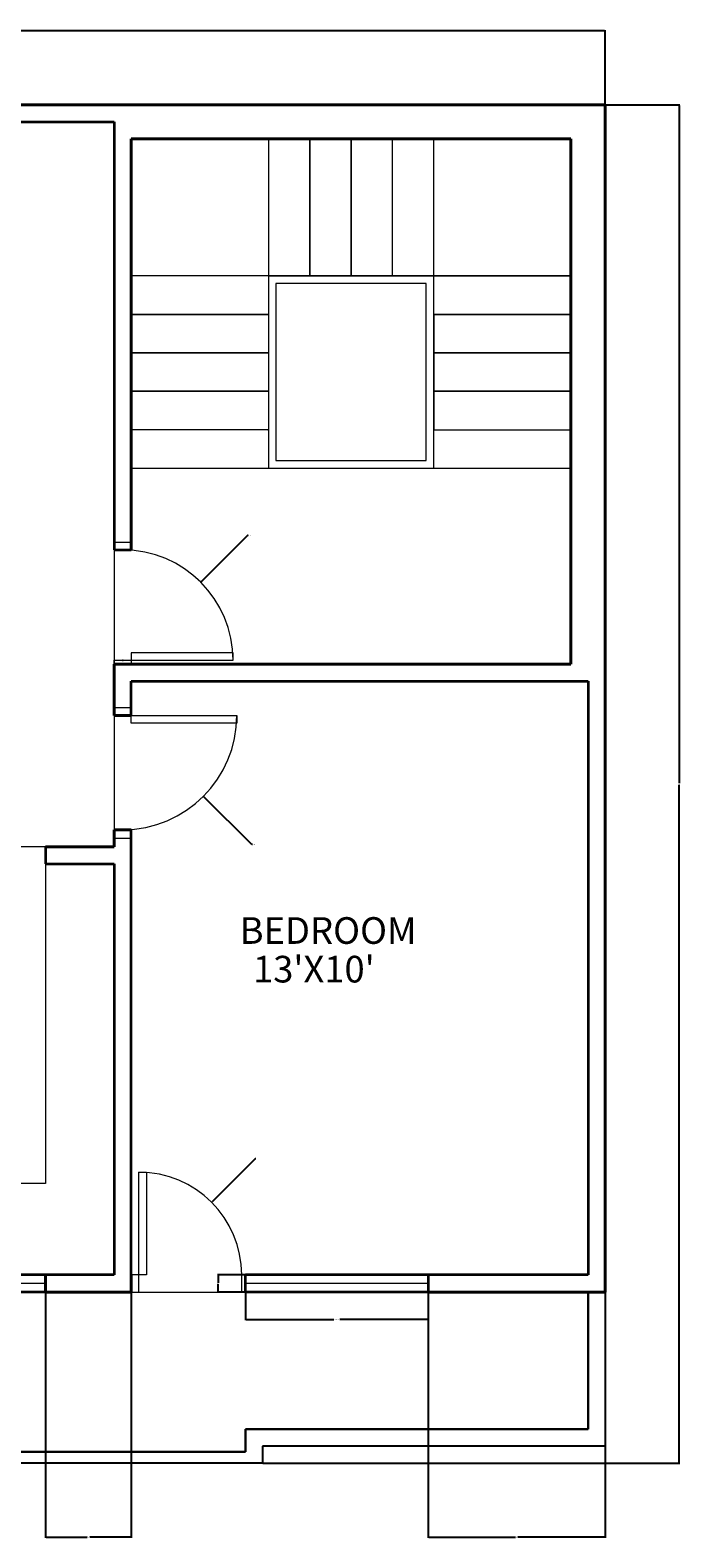
# Model space of a CAD drawing. Units: millimetres. Extents: x 2284 to 2706, y 1197 to 2041.
# Tile 2 of 3: x 2535 to 2706, y 1197 to 1593. Entities that reach past the tile are written whole.
import ezdxf

# ---------------------------------------------------------------- set-up
doc = ezdxf.new("R2010")
doc.units = ezdxf.units.MM
for name, color, linetype, lineweight in [('A-ANNO-DIMS', 2, 'Continuous', 18), ('A-AREA-IDEN', 7, 'Continuous', 30), ('A-CONS', 67, 'Continuous', 13), ('A-DOOR', 7, 'Continuous', 18), ('A-FLOR-FIXT', 6, 'Continuous', 18)]:
    doc.layers.add(name, color=color, linetype=linetype, lineweight=lineweight)
for name, color, linetype, lineweight, true_color in [('A-FLOR-STRS', 67, 'Continuous', 18, 0x727430), ('A-GLAZ', 219, 'Continuous', 18, 0x642165), ('A-WALL', 11, 'Continuous', 35, 0xf27172), ('A-WALL-PRPT', 143, 'Continuous', 25, 0x7aafdf)]:
    doc.layers.add(name, color=color, linetype=linetype, lineweight=lineweight, true_color=true_color)
doc.styles.get("Standard").update_dxf_attribs({"font": 'arial.ttf'})
doc.dimstyles.get("Standard").update_dxf_attribs({"dimtxt": 0.18, "dimasz": 0.18, "dimexe": 0.18, "dimexo": 0.0625, "dimgap": 0.09, "dimtad": 0, "dimtih": 1, "dimtoh": 1, "dimdec": 4, "dimzin": 0, "dimdsep": 46, "dimtxsty": 'Standard', "dimcen": 0.09, "dimadec": 0, "dimazin": 0, "dimtfac": 1, "dimtdec": 4, "dimtofl": 0, "dimtmove": 0, "dimatfit": 3, "dimfxl": 1, "dimtolj": 1, "dimtzin": 0, "dimarcsym": 0})

# ---------------------------------------------------------------- blocks, each defined once
blk = doc.blocks.new('STAIR-U-RETURN')
for p, q in [((0, 86.5), (36, 86.5)), ((36, 86.5), (36, 50.5)), ((46.87, 50.5), (46.87, 86.5)), ((46.87, 86.5), (46.87, 50.5)), ((57.75, 50.5), (57.75, 86.5)), ((57.75, 86.5), (57.75, 50.5)), ((68.62, 50.5), (68.62, 86.5)), ((79.5, 50.5), (79.5, 86.5)), ((115.5, 50.5), (0, 50.5)), ((36, 50.5), (36, 0)), ((36, 50.5), (79.5, 50.5)), ((38, 48.5), (38, 2)), ((77.5, 48.5), (38, 48.5)), ((77.5, 2), (77.5, 48.5)), ((79.5, 0), (79.5, 50.5)), ((36, 40.4), (0, 40.4)), ((0, 40.4), (36, 40.4)), ((36, 40.4), (36, 30.3)), ((79.5, 40.4), (79.5, 30.3)), ((79.5, 40.4), (115.5, 40.4)), ((115.5, 40.4), (79.5, 40.4)), ((36, 30.3), (0, 30.3)), ((0, 30.3), (36, 30.3)), ((36, 30.3), (36, 20.2)), ((79.5, 30.3), (79.5, 20.2)), ((79.5, 30.3), (115.5, 30.3)), ((115.5, 30.3), (79.5, 30.3)), ((36, 20.2), (0, 20.2)), ((0, 20.2), (36, 20.2)), ((36, 20.2), (36, 10.1)), ((79.5, 20.2), (79.5, 10.1)), ((79.5, 20.2), (115.5, 20.2)), ((115.5, 20.2), (79.5, 20.2)), ((36, 10.1), (0, 10.1)), ((79.5, 10.1), (115.5, 10.1)), ((0, 0), (115.5, 0)), ((38, 2), (77.5, 2))]:
    blk.add_line(p, q)
blk = doc.blocks.new('WIN-36')
for p, q in [((36, 4.5), (0, 4.5)), ((0, 4.5), (0, 0)), ((36, 0), (36, 4.5)), ((36, 2.25), (0, 2.25)), ((0, 0), (36, 0)), ((36, 0), (36, 2.25))]:
    blk.add_line(p, q)
blk = doc.blocks.new('WIN-48')
for p, q in [((4.5, 48), (0, 48)), ((0, 48), (0, 0)), ((2.25, 0), (2.25, 48)), ((4.5, 0), (4.5, 48)), ((0, 0), (4.5, 0)), ((0, 0), (2.25, 0))]:
    blk.add_line(p, q)
blk = doc.blocks.new('*D15')
at = {"layer": 'A-ANNO-DIMS', "color": 0, "lineweight": -2, "transparency": 16777216}
for p, q in [((2591.45, 1261.24), (2591.45, 1253.92)), ((2639.45, 1261.24), (2639.45, 1253.92)), ((2591.63, 1254.1), (2614.7, 1254.1)), ((2639.27, 1254.1), (2616.21, 1254.1))]:
    blk.add_line(p, q, dxfattribs=at)
at = {"layer": 'A-ANNO-DIMS', "color": 0, "transparency": 16777216}
for points in [[(2591.63, 1254.13), (2591.63, 1254.07), (2591.45, 1254.1)], [(2639.27, 1254.13), (2639.27, 1254.07), (2639.45, 1254.1)]]:
    blk.add_solid(points, dxfattribs=at)
at = {"layer": 'Defpoints', "color": 0, "transparency": 16777216}
for p in [(2591.45, 1261.3), (2639.45, 1261.3), (2591.45, 1254.1)]:
    blk.add_point(p, dxfattribs=at)
at = {"layer": 'A-ANNO-DIMS', "color": 0, "transparency": 16777216, "insert": (2615.45, 1254.1), "char_height": 0.18, "attachment_point": 5}
blk.add_mtext('\\A1;W3 48 TYP.', dxfattribs=at)
blk = doc.blocks.new('*D16')
at = {"layer": 'A-ANNO-DIMS', "color": 0, "lineweight": -2, "transparency": 16777216}
for p, q in [((2591.39, 1265.8), (2584.07, 1265.8)), ((2584.25, 1265.62), (2584.25, 1263.73)), ((2591.39, 1261.3), (2584.07, 1261.3)), ((2584.25, 1261.48), (2584.25, 1263.37))]:
    blk.add_line(p, q, dxfattribs=at)
at = {"layer": 'A-ANNO-DIMS', "color": 0, "transparency": 16777216}
for points in [[(2584.22, 1265.62), (2584.28, 1265.62), (2584.25, 1265.8)], [(2584.22, 1261.48), (2584.28, 1261.48), (2584.25, 1261.3)]]:
    blk.add_solid(points, dxfattribs=at)
at = {"layer": 'Defpoints', "color": 0, "transparency": 16777216}
for p in [(2584.25, 1265.8), (2591.45, 1265.8), (2591.45, 1261.3)]:
    blk.add_point(p, dxfattribs=at)
at = {"layer": 'A-ANNO-DIMS', "color": 0, "transparency": 16777216, "insert": (2584.25, 1263.55), "char_height": 0.18, "attachment_point": 5}
blk.add_mtext('\\A1;5 TYP.', dxfattribs=at)
blk = doc.blocks.new('*D28')
at = {"layer": 'A-ANNO-DIMS', "color": 0, "lineweight": -2, "transparency": 16777216}
for p, q in [((2310.95, 1483.36), (2310.95, 1592.88)), ((2311.13, 1592.7), (2498.17, 1592.7)), ((2685.77, 1592.7), (2498.74, 1592.7)), ((2685.95, 1573.36), (2685.95, 1592.88))]:
    blk.add_line(p, q, dxfattribs=at)
at = {"layer": 'A-ANNO-DIMS', "color": 0, "transparency": 16777216}
for points in [[(2311.13, 1592.73), (2311.13, 1592.67), (2310.95, 1592.7)], [(2685.77, 1592.73), (2685.77, 1592.67), (2685.95, 1592.7)]]:
    blk.add_solid(points, dxfattribs=at)
at = {"layer": 'Defpoints', "color": 0, "transparency": 16777216}
for p in [(2685.95, 1592.7), (2685.95, 1573.3), (2310.95, 1483.3)]:
    blk.add_point(p, dxfattribs=at)
at = {"layer": 'A-ANNO-DIMS', "color": 0, "transparency": 16777216, "insert": (2498.45, 1592.7), "char_height": 0.18, "attachment_point": 5}
blk.add_mtext('\\A1;375', dxfattribs=at)
blk = doc.blocks.new('*D29')
at = {"layer": 'A-ANNO-DIMS', "color": 0, "lineweight": -2, "transparency": 16777216}
for p, q in [((2686.02, 1573.3), (2705.53, 1573.3)), ((2705.35, 1573.12), (2705.35, 1394.98)), ((2705.35, 1216.48), (2705.35, 1394.62)), ((2596.02, 1216.3), (2705.53, 1216.3))]:
    blk.add_line(p, q, dxfattribs=at)
at = {"layer": 'A-ANNO-DIMS', "color": 0, "transparency": 16777216}
for points in [[(2705.32, 1573.12), (2705.38, 1573.12), (2705.35, 1573.3)], [(2705.32, 1216.48), (2705.38, 1216.48), (2705.35, 1216.3)]]:
    blk.add_solid(points, dxfattribs=at)
at = {"layer": 'Defpoints', "color": 0, "transparency": 16777216}
for p in [(2685.95, 1573.3), (2705.35, 1573.3), (2595.95, 1216.3)]:
    blk.add_point(p, dxfattribs=at)
at = {"layer": 'A-ANNO-DIMS', "color": 0, "transparency": 16777216, "insert": (2705.35, 1394.8), "char_height": 0.18, "attachment_point": 5}
blk.add_mtext('\\A1;357', dxfattribs=at)
blk = doc.blocks.new('*D36')
at = {"layer": 'A-ANNO-DIMS', "color": 0, "lineweight": -2, "transparency": 16777216}
for p, q in [((2538.95, 1261.24), (2538.95, 1196.72)), ((2561.45, 1261.24), (2561.45, 1196.72)), ((2539.13, 1196.9), (2549.88, 1196.9)), ((2561.27, 1196.9), (2550.53, 1196.9))]:
    blk.add_line(p, q, dxfattribs=at)
at = {"layer": 'A-ANNO-DIMS', "color": 0, "transparency": 16777216}
for points in [[(2539.13, 1196.93), (2539.13, 1196.87), (2538.95, 1196.9)], [(2561.27, 1196.93), (2561.27, 1196.87), (2561.45, 1196.9)]]:
    blk.add_solid(points, dxfattribs=at)
at = {"layer": 'Defpoints', "color": 0, "transparency": 16777216}
for p in [(2538.95, 1261.3), (2561.45, 1261.3), (2561.45, 1196.9)]:
    blk.add_point(p, dxfattribs=at)
at = {"layer": 'A-ANNO-DIMS', "color": 0, "transparency": 16777216, "insert": (2550.2, 1196.9), "char_height": 0.18, "attachment_point": 5}
blk.add_mtext('\\A1;22.5', dxfattribs=at)
blk = doc.blocks.new('*D37')
at = {"layer": 'A-ANNO-DIMS', "color": 0, "lineweight": -2, "transparency": 16777216}
for p, q in [((2639.45, 1261.24), (2639.45, 1196.72)), ((2685.95, 1261.24), (2685.95, 1196.72)), ((2639.63, 1196.9), (2662.38, 1196.9)), ((2685.77, 1196.9), (2663.03, 1196.9))]:
    blk.add_line(p, q, dxfattribs=at)
at = {"layer": 'A-ANNO-DIMS', "color": 0, "transparency": 16777216}
for points in [[(2639.63, 1196.93), (2639.63, 1196.87), (2639.45, 1196.9)], [(2685.77, 1196.93), (2685.77, 1196.87), (2685.95, 1196.9)]]:
    blk.add_solid(points, dxfattribs=at)
at = {"layer": 'Defpoints', "color": 0, "transparency": 16777216}
for p in [(2639.45, 1261.3), (2685.95, 1261.3), (2685.95, 1196.9)]:
    blk.add_point(p, dxfattribs=at)
at = {"layer": 'A-ANNO-DIMS', "color": 0, "transparency": 16777216, "insert": (2662.7, 1196.9), "char_height": 0.18, "attachment_point": 5}
blk.add_mtext('\\A1;46.5', dxfattribs=at)
blk = doc.blocks.new('*D39')
at = {"layer": 'A-ANNO-DIMS', "color": 0, "lineweight": -2, "transparency": 16777216}
for p, q in [((2559.11, 1412.8), (2559.29, 1412.8)), ((2559.2, 1412.71), (2559.2, 1412.89)), ((2593.15, 1378.86), (2580.55, 1391.46)), ((2593.33, 1378.86), (2593.15, 1378.86))]:
    blk.add_line(p, q, dxfattribs=at)
at = {"layer": 'A-ANNO-DIMS', "color": 0, "transparency": 16777216}
blk.add_solid([(2580.57, 1391.48), (2580.52, 1391.44), (2580.42, 1391.59)], dxfattribs=at)
at = {"layer": 'Defpoints', "color": 0, "transparency": 16777216}
for p in [(2559.2, 1412.8), (2580.42, 1391.59)]:
    blk.add_point(p, dxfattribs=at)
at = {"layer": 'A-ANNO-DIMS', "color": 0, "transparency": 16777216, "insert": (2593.63, 1378.86), "char_height": 0.18, "attachment_point": 5}
blk.add_mtext('\\A1;R30', dxfattribs=at)
blk = doc.blocks.new('*D40')
at = {"layer": 'A-ANNO-DIMS', "color": 0, "lineweight": -2, "transparency": 16777216}
for p, q in [((2592.01, 1460.11), (2579.84, 1447.93)), ((2592.19, 1460.11), (2592.01, 1460.11)), ((2559.11, 1427.3), (2559.29, 1427.3)), ((2559.2, 1427.21), (2559.2, 1427.39))]:
    blk.add_line(p, q, dxfattribs=at)
at = {"layer": 'A-ANNO-DIMS', "color": 0, "transparency": 16777216}
blk.add_solid([(2579.82, 1447.95), (2579.86, 1447.91), (2579.71, 1447.81)], dxfattribs=at)
at = {"layer": 'Defpoints', "color": 0, "transparency": 16777216}
for p in [(2579.71, 1447.81), (2559.2, 1427.3)]:
    blk.add_point(p, dxfattribs=at)
at = {"layer": 'A-ANNO-DIMS', "color": 0, "transparency": 16777216, "insert": (2592.5, 1460.11), "char_height": 0.18, "attachment_point": 5}
blk.add_mtext('\\A1;R29', dxfattribs=at)
blk = doc.blocks.new('*D41')
at = {"layer": 'A-ANNO-DIMS', "color": 0, "lineweight": -2, "transparency": 16777216}
for p, q in [((2594, 1296.35), (2582.67, 1285.02)), ((2594.18, 1296.35), (2594, 1296.35)), ((2563.36, 1265.8), (2563.54, 1265.8)), ((2563.45, 1265.71), (2563.45, 1265.89))]:
    blk.add_line(p, q, dxfattribs=at)
at = {"layer": 'A-ANNO-DIMS', "color": 0, "transparency": 16777216}
blk.add_solid([(2582.65, 1285.04), (2582.7, 1285), (2582.55, 1284.89)], dxfattribs=at)
at = {"layer": 'Defpoints', "color": 0, "transparency": 16777216}
for p in [(2582.55, 1284.89), (2563.45, 1265.8)]:
    blk.add_point(p, dxfattribs=at)
at = {"layer": 'A-ANNO-DIMS', "color": 0, "transparency": 16777216, "insert": (2594.49, 1296.35), "char_height": 0.18, "attachment_point": 5}
blk.add_mtext('\\A1;R27', dxfattribs=at)

msp = doc.modelspace()

# ---------------------------------------------------------------- linework, layer by layer
at = {"layer": 'A-CONS'}
for p in [(2608.33, 1528.3), (2619.2, 1528.3), (2630.08, 1528.3), (2597.45, 1518.2), (2640.95, 1518.2), (2597.45, 1508.1), (2640.95, 1508.1), (2597.45, 1498), (2640.95, 1498), (2597.45, 1487.9), (2640.95, 1487.9)]:
    msp.add_point(p, dxfattribs=at)
at = {"layer": 'A-DOOR'}
for p, q in [((2561.45, 1458.3), (2556.95, 1458.3)), ((2556.95, 1458.3), (2556.95, 1456.3)), ((2561.45, 1456.3), (2561.45, 1458.3)), ((2556.95, 1456.3), (2561.45, 1456.3)), ((2556.95, 1456.3), (2556.95, 1426.3)), ((2556.95, 1426.3), (2556.95, 1427.3)), ((2556.95, 1427.3), (2561.45, 1427.3)), ((2561.45, 1426.3), (2556.95, 1426.3)), ((2588.2, 1429.3), (2561.45, 1429.3)), ((2561.45, 1429.3), (2561.45, 1427.3)), ((2561.45, 1427.3), (2561.45, 1426.3)), ((2561.45, 1427.3), (2588.2, 1427.3)), ((2588.2, 1427.3), (2588.2, 1429.3)), ((2561.45, 1414.8), (2556.95, 1414.8)), ((2556.95, 1414.8), (2556.95, 1412.8)), ((2561.45, 1412.8), (2561.45, 1414.8)), ((2556.95, 1412.8), (2556.95, 1382.8)), ((2556.95, 1412.8), (2561.45, 1412.8)), ((2556.95, 1412.8), (2561.45, 1412.8)), ((2561.45, 1412.8), (2589.2, 1412.8)), ((2561.45, 1410.8), (2561.45, 1412.8)), ((2589.2, 1410.8), (2561.45, 1410.8)), ((2589.2, 1412.8), (2589.2, 1410.8)), ((2556.95, 1382.8), (2556.95, 1380.55)), ((2561.45, 1382.8), (2556.95, 1382.8)), ((2561.45, 1380.55), (2561.45, 1382.8)), ((2556.95, 1380.55), (2561.45, 1380.55)), ((2563.45, 1265.8), (2563.45, 1292.8)), ((2563.45, 1292.8), (2565.45, 1292.8)), ((2565.45, 1292.8), (2565.45, 1265.8)), ((2563.45, 1265.8), (2561.45, 1265.8)), ((2561.45, 1265.8), (2561.45, 1261.3)), ((2563.45, 1261.3), (2563.45, 1265.8)), ((2565.45, 1265.8), (2563.45, 1265.8)), ((2590.45, 1261.3), (2590.45, 1265.8)), ((2590.45, 1265.8), (2591.45, 1265.8)), ((2561.45, 1261.3), (2563.45, 1261.3)), ((2563.45, 1261.3), (2591.45, 1261.3)), ((2591.45, 1261.3), (2590.45, 1261.3))]:
    msp.add_line(p, q, dxfattribs=at)
for centre, radius, start, end in [((2559.2, 1427.3), 29, 0, 90), ((2559.2, 1412.8), 30, 270, 0), ((2563.45, 1265.8), 27, 0, 90)]:
    msp.add_arc(centre, radius, start, end, dxfattribs=at)
at = {"layer": 'A-FLOR-FIXT'}
for p, q in [((2538.95, 1378.3), (2484.95, 1378.3)), ((2538.95, 1373.8), (2538.95, 1289.8)), ((2538.95, 1289.8), (2484.95, 1289.8))]:
    msp.add_line(p, q, dxfattribs=at)
at = {"layer": 'A-FLOR-STRS'}
for p, q in [((2597.45, 1528.3), (2676.95, 1528.3)), ((2676.95, 1528.3), (2640.95, 1528.3)), ((2597.45, 1477.8), (2676.95, 1477.8))]:
    msp.add_line(p, q, dxfattribs=at)
at = {"layer": 'A-GLAZ'}
for p, q in [((2591.45, 1265.8), (2639.45, 1265.8)), ((2502.95, 1261.3), (2538.95, 1261.3))]:
    msp.add_line(p, q, dxfattribs=at)
at = {"layer": 'A-WALL'}
for p, q in [((2355.95, 1573.3), (2685.95, 1573.3)), ((2685.95, 1573.3), (2355.95, 1573.3)), ((2685.95, 1573.3), (2676.95, 1573.3)), ((2685.95, 1573.3), (2685.95, 1261.3)), ((2685.95, 1261.3), (2685.95, 1573.3)), ((2360.45, 1568.8), (2556.95, 1568.8)), ((2424.95, 1568.8), (2556.95, 1568.8)), ((2556.95, 1568.8), (2556.95, 1456.3)), ((2556.95, 1568.8), (2556.95, 1456.3)), ((2676.95, 1564.3), (2561.45, 1564.3)), ((2561.45, 1564.3), (2561.45, 1456.3)), ((2561.45, 1456.3), (2561.45, 1564.3)), ((2561.45, 1564.3), (2676.95, 1564.3)), ((2676.95, 1426.3), (2676.95, 1564.3)), ((2676.95, 1564.3), (2676.95, 1426.3)), ((2556.95, 1456.3), (2561.45, 1456.3)), ((2556.95, 1456.3), (2561.45, 1456.3)), ((2556.95, 1426.3), (2561.45, 1426.3)), ((2556.95, 1412.8), (2556.95, 1426.3)), ((2676.95, 1426.3), (2556.95, 1426.3)), ((2556.95, 1426.3), (2556.95, 1412.8)), ((2561.45, 1426.3), (2676.95, 1426.3)), ((2561.45, 1421.8), (2681.45, 1421.8)), ((2561.45, 1412.8), (2561.45, 1421.8)), ((2561.45, 1412.8), (2561.45, 1421.8)), ((2561.45, 1421.8), (2681.45, 1421.8)), ((2561.45, 1412.8), (2561.45, 1421.8)), ((2681.45, 1421.8), (2681.45, 1265.8)), ((2681.45, 1421.8), (2681.45, 1265.8)), ((2556.95, 1412.8), (2561.45, 1412.8)), ((2561.45, 1412.8), (2556.95, 1412.8)), ((2556.95, 1412.8), (2561.45, 1412.8)), ((2556.95, 1378.3), (2556.95, 1382.8)), ((2556.95, 1382.8), (2561.45, 1382.8)), ((2561.45, 1382.8), (2556.95, 1382.8)), ((2556.95, 1382.8), (2556.95, 1378.3)), ((2561.45, 1265.8), (2561.45, 1382.8)), ((2561.45, 1261.3), (2561.45, 1382.8)), ((2538.95, 1378.3), (2556.95, 1378.3)), ((2556.95, 1378.3), (2538.95, 1378.3)), ((2538.95, 1378.3), (2538.95, 1373.8)), ((2538.95, 1373.8), (2556.95, 1373.8)), ((2538.95, 1373.8), (2556.95, 1373.8)), ((2556.95, 1373.8), (2556.95, 1265.8)), ((2556.95, 1373.8), (2556.95, 1265.8)), ((2556.95, 1265.8), (2484.95, 1265.8)), ((2538.95, 1261.3), (2538.95, 1265.8)), ((2538.95, 1265.8), (2538.95, 1261.3)), ((2556.95, 1265.8), (2538.95, 1265.8)), ((2561.45, 1265.8), (2561.45, 1261.3)), ((2681.45, 1265.8), (2591.45, 1265.8)), ((2591.45, 1261.3), (2591.45, 1265.8)), ((2639.45, 1265.8), (2639.45, 1261.3)), ((2681.45, 1265.8), (2639.45, 1265.8)), ((2639.45, 1265.8), (2639.45, 1261.3)), ((2561.45, 1261.3), (2355.95, 1261.3)), ((2538.95, 1261.3), (2561.45, 1261.3)), ((2685.95, 1261.3), (2591.45, 1261.3)), ((2639.45, 1261.3), (2685.95, 1261.3)), ((2685.95, 1261.3), (2681.45, 1261.3))]:
    msp.add_line(p, q, dxfattribs=at)
at = {"layer": 'A-WALL-PRPT'}
for p, q in [((2681.45, 1261.3), (2681.45, 1225.3)), ((2681.45, 1225.3), (2681.45, 1261.3)), ((2685.95, 1261.3), (2685.95, 1225.3)), ((2685.95, 1261.3), (2685.95, 1220.8)), ((2681.45, 1225.3), (2591.45, 1225.3)), ((2591.45, 1225.3), (2591.45, 1219.3)), ((2591.45, 1219.3), (2591.45, 1225.3)), ((2591.45, 1225.3), (2681.45, 1225.3)), ((2685.95, 1225.3), (2685.95, 1220.8)), ((2685.95, 1220.8), (2595.95, 1220.8)), ((2595.95, 1220.8), (2595.95, 1216.3)), ((2685.95, 1220.8), (2595.95, 1220.8)), ((2595.95, 1220.8), (2595.95, 1216.3)), ((2595.95, 1216.3), (2405.45, 1216.3)), ((2591.45, 1219.3), (2409.95, 1219.3)), ((2409.95, 1219.3), (2591.45, 1219.3)), ((2595.95, 1216.3), (2409.95, 1216.3))]:
    msp.add_line(p, q, dxfattribs=at)

# ---------------------------------------------------------------- block references
at = {"layer": 'A-FLOR-STRS'}
msp.add_blockref('STAIR-U-RETURN', (2561.46, 1477.8), dxfattribs=at)
at = {"layer": 'A-GLAZ', "extrusion": (0, 0, -1), "zscale": -1, "rotation": 180}
msp.add_blockref('WIN-36', (-2502.95, 1265.8), dxfattribs=at)
at = {"layer": 'A-GLAZ', "rotation": 90.00000000000087}
msp.add_blockref('WIN-48', (2639.45, 1261.3), dxfattribs=at)

# ---------------------------------------------------------------- texts
at = {"layer": 'A-AREA-IDEN'}
for s, p in [('BEDROOM', (2589.93, 1352.8)), ("13'X10'", (2593.43, 1342.65))]:
    msp.add_text(s, height=7, dxfattribs=at).set_placement(p)

# ---------------------------------------------------------------- dimensions: what is measured, and where the dimension line sits
at = {"layer": 'A-ANNO-DIMS'}
for base, p1, p2, override, picture, middle in [((2685.95, 1592.7), (2310.95, 1483.3), (2685.95, 1573.3), {"dimdec": 0, "dimlfac": 1, "dimrnd": 0, "dimzin": 0, "dimdsep": 46, "dimlunit": 2}, '*D28', (2498.45, 1592.7)), ((2561.45, 1196.9), (2538.95, 1261.3), (2561.45, 1261.3), {"dimdec": 1, "dimlfac": 1, "dimrnd": 0, "dimzin": 0, "dimdsep": 46, "dimlunit": 2}, '*D36', (2550.2, 1196.9)), ((2685.95, 1196.9), (2639.45, 1261.3), (2685.95, 1261.3), {"dimdec": 1, "dimlfac": 1, "dimrnd": 0, "dimzin": 0, "dimdsep": 46, "dimlunit": 2}, '*D37', (2662.7, 1196.9))]:
    dim = msp.add_linear_dim(base=base, p1=p1, p2=p2, dimstyle='Standard', override=override, dxfattribs=at)
    dim.commit()
    dim.dimension.update_dxf_attribs({"geometry": picture, "text_midpoint": middle})
dim = msp.add_linear_dim(base=(2705.35, 1573.3), p1=(2595.95, 1216.3), p2=(2685.95, 1573.3), angle=90, dimstyle='Standard', override={"dimdec": 0, "dimlfac": 1, "dimrnd": 0, "dimzin": 0, "dimdsep": 46, "dimlunit": 2}, dxfattribs=at)
dim.commit()
dim.dimension.update_dxf_attribs({"geometry": '*D29', "text_midpoint": (2705.35, 1394.8)})
for center, mpoint, picture, middle in [((2559.2, 1427.3), (2579.71, 1447.81), '*D40', (2592.5, 1460.11)), ((2559.2, 1412.8), (2580.42, 1391.59), '*D39', (2593.63, 1378.86)), ((2563.45, 1265.8), (2582.55, 1284.89), '*D41', (2594.49, 1296.35))]:
    dim = msp.add_radius_dim(center=center, mpoint=mpoint, dimstyle='Standard', override={"dimdec": 0, "dimlfac": 1, "dimrnd": 0, "dimzin": 0, "dimdsep": 46, "dimlunit": 2}, dxfattribs=at)
    dim.commit()
    dim.dimension.update_dxf_attribs({"geometry": picture, "text_midpoint": middle, "dimtype": 164})
for base, p1, p2, angle, text, picture, middle in [((2584.25492415, 1265.80003665), (2591.45492415, 1261.30003665), (2591.45492415, 1265.80003665), 90, '<> TYP.', '*D16', (2584.25492415, 1263.55003665)), ((2591.45, 1254.1), (2639.45, 1261.3), (2591.45, 1261.3), 180, 'W3 <> TYP.', '*D15', (2615.45, 1254.1))]:
    dim = msp.add_linear_dim(base=base, p1=p1, p2=p2, angle=angle, text=text, dimstyle='Standard', override={"dimdec": 0, "dimlfac": 1, "dimrnd": 0, "dimzin": 0, "dimdsep": 46, "dimlunit": 2}, dxfattribs=at)
    dim.commit()
    dim.dimension.update_dxf_attribs({"geometry": picture, "text_midpoint": middle})

doc.saveas('drawing.dxf')
